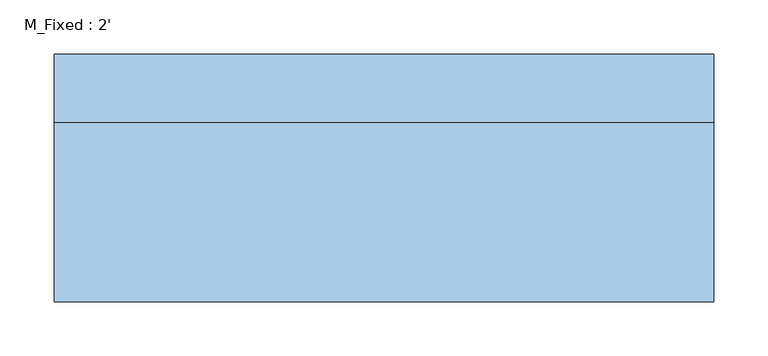
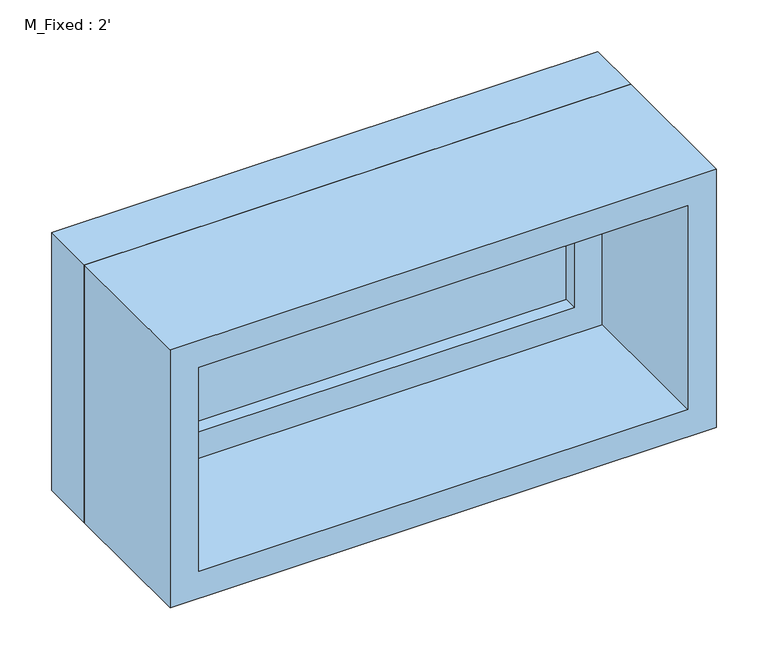
"""IFC4 building model written with IfcOpenShell, lengths in millimetres: window geometry, M_Fixed : 2'."""

from ifc_helpers import new_model, si_unit, frame, origin, place, context, project, spatial, polyline, outline, extrude, source, transform, mapped, element, save


def m_fixed_2_dd9f9b20(model_context):
    return source(origin(), model_context, "Body", "SweptSolid", [
        extrude(outline(polyline([(-241.8, 92.3), (241.8, 92.3), (241.8, 80.3), (-241.8, 80.3), (-241.8, 92.3)])), frame((0.0, 0.0, 978.0), z_axis=(0.0, 0.0, 1.0), x_axis=(1.0, 0.0, 0.0)), (0.0, 0.0, 1.0), 178.8),
        extrude(outline(polyline([(1200.8, -285.8), (934.0, -285.8), (934.0, 285.8), (1200.8, 285.8), (1200.8, -285.8)]), holes=[polyline([(1156.8, -241.8), (1156.8, 241.8), (978.0, 241.8), (978.0, -241.8), (1156.8, -241.8)])]), frame((0.0, 64.3, 0.0), z_axis=(0.0, 1.0, 0.0), x_axis=(0.0, 0.0, 1.0)), (0.0, 0.0, 1.0), 44.0),
        extrude(outline(polyline([(1219.8, -304.8), (915.0, -304.8), (915.0, 304.8), (1219.8, 304.8), (1219.8, -304.8)]), holes=[polyline([(1200.8, -285.8), (1200.8, 285.8), (934.0, 285.8), (934.0, -285.8), (1200.8, -285.8)])]), frame((0.0, 64.3, 0.0), z_axis=(0.0, 1.0, 0.0), x_axis=(0.0, 0.0, 1.0)), (0.0, 0.0, 1.0), 63.0),
        extrude(outline(polyline([(1219.8, -304.8), (915.0, -304.8), (915.0, 304.8), (1219.8, 304.8), (1219.8, -304.8)]), holes=[polyline([(1187.8, -272.8), (1187.8, 272.8), (947.0, 272.8), (947.0, -272.8), (1187.8, -272.8)])]), frame((0.0, -101.3, 0.0), z_axis=(0.0, 1.0, 0.0), x_axis=(0.0, 0.0, 1.0)), (0.0, 0.0, 1.0), 165.6),
    ])


if __name__ == "__main__":
    model = new_model("IFC4")
    model_context = context("Model", 3, world=origin())
    ifc_project = project(units=[si_unit("LENGTHUNIT", "METRE", prefix="MILLI")], contexts=[model_context])
    site = spatial("IfcSite", under=ifc_project)
    building = spatial("IfcBuilding", under=site)
    placement = place(None, origin())
    m_fixed_2_shape = m_fixed_2_dd9f9b20(model_context)
    element("IfcWindow", 1, ObjectType="M_Fixed : 2'", at=placement, inside=building, context=model_context, shape_type="MappedRepresentation", body=[
        mapped(m_fixed_2_shape, transform((0.0, 0.0, 0.0), x_axis=(1.0, 0.0, 0.0), y_axis=(0.0, 1.0, 0.0), z_axis=(0.0, 0.0, 1.0))),
    ])
    save(model, "model.ifc")

# Revit data of these elements
# Type "M_Fixed : 2'"
#   Type Mark = "37"
#   Construction Type Id = "GSP4R"
#   Analytic Construction = "1/8 in Pilkington single glazing"
#   Visual Light Transmittance = 0.9
#   Thermal Resistance (R) = 0.271106 (m²·K)/W
#   Solar Heat Gain Coefficient = 0.78
#   Heat Transfer Coefficient (U) = 3.6886 W/(m²·K)
#   Height = 1' - 0"
#   Default Sill Height = 3' - 0.02362"
#   Width = 2' - 0"
#   Window Inset = 0' - 0.74803"
#   Define Thermal Properties by = 1
#   Frame Exterior Material = Sash
#   Frame Interior Material = Sash
#   Glass Pane Material = Glass
#   Sash = Sash
#   Wall Closure = (empty or 0)
# Element 1 (IfcWindow, "M_Fixed : 2'")
#   Materials on its faces: "Sash", "Glass"
# Materials
#   "Sash": class "Wood", colour RGB 224 178 126, transparency 0, Cost = 0
#   "Glass": class "Glass", colour RGB 0 128 192, transparency 0.9, Description = "Soda Lime Glass", Cost = 0
